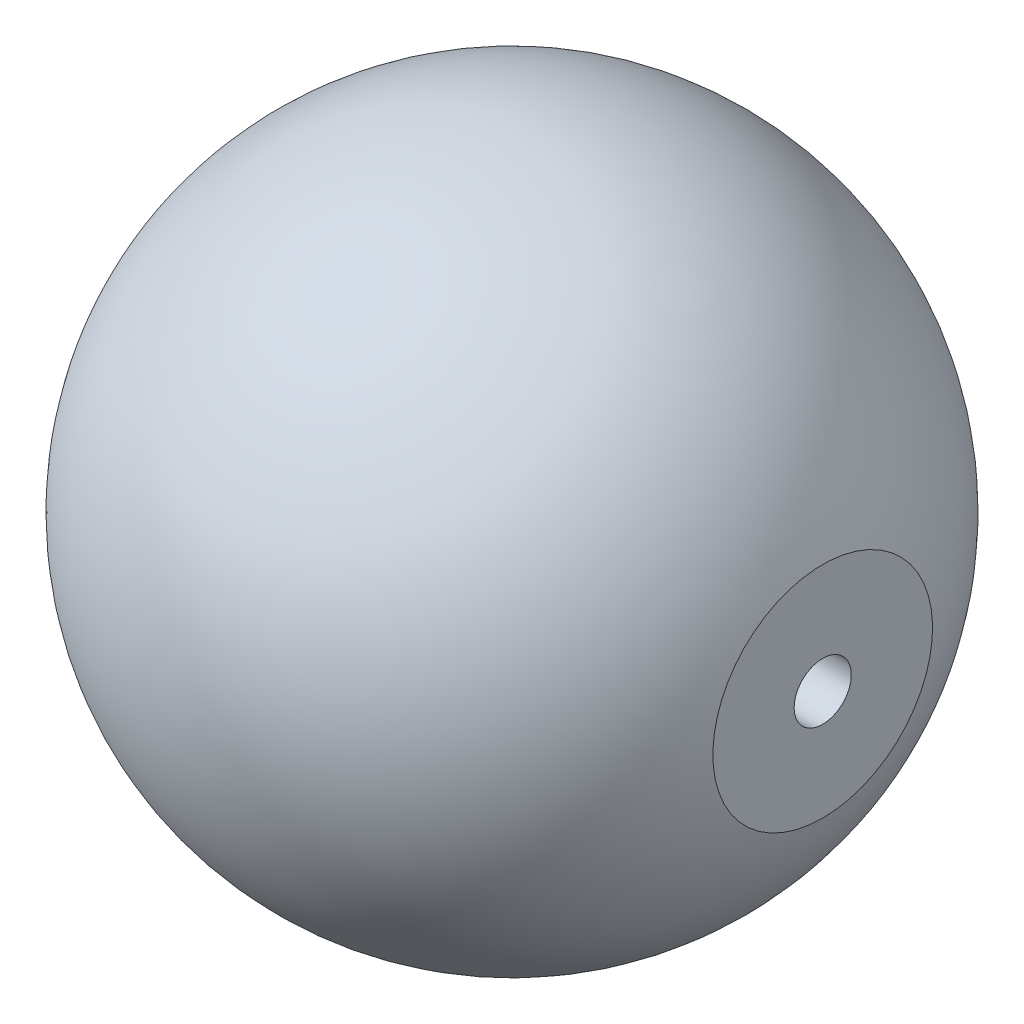
ISO-10303-21;
HEADER;
FILE_DESCRIPTION(('STEP AP214'),'2;1');
FILE_NAME('part.step','',(''),(''),'','','');
FILE_SCHEMA(('AUTOMOTIVE_DESIGN { 1 0 10303 214 1 1 1 1 }'));
ENDSEC;
DATA;
#1=APPLICATION_CONTEXT('core data for automotive mechanical design processes');
#2=APPLICATION_PROTOCOL_DEFINITION('international standard','automotive_design',2000,#1);
#3=PRODUCT_CONTEXT('',#1,'mechanical');
#4=PRODUCT('Part','Part','',(#3));
#5=PRODUCT_RELATED_PRODUCT_CATEGORY('part','',(#4));
#6=PRODUCT_DEFINITION_FORMATION('','',#4);
#7=PRODUCT_DEFINITION_CONTEXT('part definition',#1,'design');
#8=PRODUCT_DEFINITION('design','',#6,#7);
#9=PRODUCT_DEFINITION_SHAPE('','',#8);
#10=(LENGTH_UNIT() NAMED_UNIT(*) SI_UNIT(.MILLI.,.METRE.));
#11=(NAMED_UNIT(*) PLANE_ANGLE_UNIT() SI_UNIT($,.RADIAN.));
#12=(NAMED_UNIT(*) SI_UNIT($,.STERADIAN.) SOLID_ANGLE_UNIT());
#13=UNCERTAINTY_MEASURE_WITH_UNIT(LENGTH_MEASURE(1.E-05),#10,'distance_accuracy_value','');
#14=(GEOMETRIC_REPRESENTATION_CONTEXT(3) GLOBAL_UNCERTAINTY_ASSIGNED_CONTEXT((#13)) GLOBAL_UNIT_ASSIGNED_CONTEXT((#10,
#11,#12)) REPRESENTATION_CONTEXT('',''));
#15=CARTESIAN_POINT('',(0.,0.,0.));
#16=DIRECTION('',(0.,0.,1.));
#17=DIRECTION('',(1.,0.,0.));
#18=AXIS2_PLACEMENT_3D('',#15,#16,#17);
#19=CARTESIAN_POINT('',(-30.,0.,0.));
#20=DIRECTION('',(-1.,0.,0.));
#21=DIRECTION('',(0.,0.,1.));
#22=AXIS2_PLACEMENT_3D('',#19,#20,#21);
#23=CYLINDRICAL_SURFACE('',#22,2.6);
#24=CARTESIAN_POINT('',(-28.2842712474619,0.,0.));
#25=DIRECTION('',(-1.,0.,0.));
#26=DIRECTION('',(0.,0.,1.));
#27=AXIS2_PLACEMENT_3D('',#24,#25,#26);
#28=CIRCLE('',#27,2.6);
#29=CARTESIAN_POINT('',(-28.2842712474619,0.,2.6));
#30=VERTEX_POINT('',#29);
#31=EDGE_CURVE('E10',#30,#30,#28,.T.);
#32=ORIENTED_EDGE('',*,*,#31,.T.);
#33=EDGE_LOOP('',(#32));
#34=FACE_BOUND('',#33,.T.);
#35=CARTESIAN_POINT('',(28.2842712474619,0.,0.));
#36=DIRECTION('',(-1.,0.,0.));
#37=DIRECTION('',(0.,0.,1.));
#38=AXIS2_PLACEMENT_3D('',#35,#36,#37);
#39=CIRCLE('',#38,2.6);
#40=CARTESIAN_POINT('',(28.2842712474619,0.,2.6));
#41=VERTEX_POINT('',#40);
#42=EDGE_CURVE('E51',#41,#41,#39,.T.);
#43=ORIENTED_EDGE('',*,*,#42,.F.);
#44=EDGE_LOOP('',(#43));
#45=FACE_BOUND('',#44,.T.);
#46=ADVANCED_FACE('F40',(#34,#45),#23,.F.);
#47=CARTESIAN_POINT('',(-28.2842712474619,-2.6,0.));
#48=DIRECTION('',(-1.,0.,0.));
#49=DIRECTION('',(0.,0.,1.));
#50=AXIS2_PLACEMENT_3D('',#47,#48,#49);
#51=PLANE('',#50);
#52=CARTESIAN_POINT('',(-28.2842712474619,0.,0.));
#53=DIRECTION('',(-1.,0.,0.));
#54=DIRECTION('',(0.,0.,1.));
#55=AXIS2_PLACEMENT_3D('',#52,#53,#54);
#56=CIRCLE('',#55,10.);
#57=CARTESIAN_POINT('',(-28.2842712474619,-10.,0.));
#58=VERTEX_POINT('',#57);
#59=EDGE_CURVE('E43',#58,#58,#56,.T.);
#60=ORIENTED_EDGE('',*,*,#59,.T.);
#61=EDGE_LOOP('',(#60));
#62=FACE_BOUND('',#61,.T.);
#63=ORIENTED_EDGE('',*,*,#31,.F.);
#64=EDGE_LOOP('',(#63));
#65=FACE_BOUND('',#64,.T.);
#66=ADVANCED_FACE('F62',(#62,#65),#51,.T.);
#67=CARTESIAN_POINT('',(0.,0.,0.));
#68=DIRECTION('',(-1.,0.,0.));
#69=DIRECTION('',(0.,-1.,0.));
#70=AXIS2_PLACEMENT_3D('',#67,#68,#69);
#71=SPHERICAL_SURFACE('',#70,30.);
#72=CARTESIAN_POINT('',(28.2842712474619,0.,0.));
#73=DIRECTION('',(-1.,0.,0.));
#74=DIRECTION('',(0.,0.,1.));
#75=AXIS2_PLACEMENT_3D('',#72,#73,#74);
#76=CIRCLE('',#75,10.);
#77=CARTESIAN_POINT('',(28.2842712474619,-10.,0.));
#78=VERTEX_POINT('',#77);
#79=EDGE_CURVE('E50',#78,#78,#76,.T.);
#80=CARTESIAN_POINT('',(28.2842712474619,-10.,0.));
#81=CARTESIAN_POINT('',(28.1560499634167,-10.3626763441463,0.));
#82=CARTESIAN_POINT('',(28.02084589577,-10.7228836236924,0.));
#83=CARTESIAN_POINT('',(27.7366882806497,-11.4378334803499,0.));
#84=CARTESIAN_POINT('',(27.5877347331762,-11.7925760574612,0.));
#85=CARTESIAN_POINT('',(27.2762942457787,-12.4960699360148,0.));
#86=CARTESIAN_POINT('',(27.1138073058547,-12.8448212374571,0.));
#87=CARTESIAN_POINT('',(26.7755415954182,-13.5358170223894,0.));
#88=CARTESIAN_POINT('',(26.5997628249058,-13.8780615058794,0.));
#89=CARTESIAN_POINT('',(26.2351732206984,-14.5555371593778,0.));
#90=CARTESIAN_POINT('',(26.0463623870035,-14.8907683293863,0.));
#91=CARTESIAN_POINT('',(25.6559880969787,-15.5537213925891,0.));
#92=CARTESIAN_POINT('',(25.4544246406489,-15.8814432857834,0.));
#93=CARTESIAN_POINT('',(25.0388433093674,-16.5288929008077,0.));
#94=CARTESIAN_POINT('',(24.8248254344156,-16.8486206226378,0.));
#95=CARTESIAN_POINT('',(24.3846519251196,-17.4796088394449,0.));
#96=CARTESIAN_POINT('',(24.1584962907753,-17.7908693344219,0.));
#97=CARTESIAN_POINT('',(23.6943818729949,-18.4044625668518,0.));
#98=CARTESIAN_POINT('',(23.4564230895589,-18.7067953043047,0.));
#99=CARTESIAN_POINT('',(22.9690544494358,-19.3020857010117,0.));
#100=CARTESIAN_POINT('',(22.7196445927487,-19.5950433602658,0.));
#101=CARTESIAN_POINT('',(22.2097428240276,-20.1711501507206,0.));
#102=CARTESIAN_POINT('',(21.9492509119935,-20.4542992819213,0.));
#103=CARTESIAN_POINT('',(21.4175704472448,-21.0103700788239,0.));
#104=CARTESIAN_POINT('',(21.1463818945302,-21.2832917445257,0.));
#105=CARTESIAN_POINT('',(20.5937093894201,-21.8185038051668,0.));
#106=CARTESIAN_POINT('',(20.3122254370247,-22.080794200106,0.));
#107=CARTESIAN_POINT('',(19.739378606273,-22.5943556436147,0.));
#108=CARTESIAN_POINT('',(19.4480157279167,-22.8456266921843,0.));
#109=CARTESIAN_POINT('',(18.8558421354703,-23.3367776711817,0.));
#110=CARTESIAN_POINT('',(18.5550314213803,-23.5766576016095,0.));
#111=CARTESIAN_POINT('',(17.9444072263787,-24.0446714264476,0.));
#112=CARTESIAN_POINT('',(17.6345937454672,-24.2728053208579,0.));
#113=CARTESIAN_POINT('',(17.0064224059104,-24.7169895348056,0.));
#114=CARTESIAN_POINT('',(16.6880645472651,-24.9330398543429,0.));
#115=CARTESIAN_POINT('',(16.0432754832885,-25.3527372581198,0.));
#116=CARTESIAN_POINT('',(15.7168442779571,-25.5563843423593,0.));
#117=CARTESIAN_POINT('',(15.0563914966943,-25.9509739665048,0.));
#118=CARTESIAN_POINT('',(14.722369920763,-26.1419165064108,0.));
#119=CARTESIAN_POINT('',(14.0472306048311,-26.5108145300486,0.));
#120=CARTESIAN_POINT('',(13.7061128648305,-26.6887700137805,0.));
#121=CARTESIAN_POINT('',(13.0172859265244,-27.0314306284194,0.));
#122=CARTESIAN_POINT('',(12.6695767282189,-27.1961357593265,0.));
#123=CARTESIAN_POINT('',(11.9680813315563,-27.5120519764192,0.));
#124=CARTESIAN_POINT('',(11.6142951331993,-27.6632630626049,0.));
#125=CARTESIAN_POINT('',(10.9011691860019,-27.9519674636707,0.));
#126=CARTESIAN_POINT('',(10.5418294371615,-28.0894607785507,0.));
#127=CARTESIAN_POINT('',(9.81812805540266,-28.3505262067507,0.));
#128=CARTESIAN_POINT('',(9.45376642248421,-28.4740983200707,0.));
#129=CARTESIAN_POINT('',(8.72056036917696,-28.7071385122147,0.));
#130=CARTESIAN_POINT('',(8.35171594878817,-28.8166065910387,0.));
#131=CARTESIAN_POINT('',(7.61009004972202,-29.0212767490864,0.));
#132=CARTESIAN_POINT('',(7.23730857104466,-29.11647882831,0.));
#133=CARTESIAN_POINT('',(6.48836010971561,-29.2924761295216,0.));
#134=CARTESIAN_POINT('',(6.11219312706391,-29.3732713515096,0.));
#135=CARTESIAN_POINT('',(5.35703022117255,-29.5203353964921,0.));
#136=CARTESIAN_POINT('',(4.97803429793287,-29.5866042194866,0.));
#137=CARTESIAN_POINT('',(4.21777425985254,-29.7045174174715,0.));
#138=CARTESIAN_POINT('',(3.83651014501188,-29.7561617924618,0.));
#139=CARTESIAN_POINT('',(3.07227782865276,-29.8447496832443,0.));
#140=CARTESIAN_POINT('',(2.6893096271343,-29.8816931990365,0.));
#141=CARTESIAN_POINT('',(1.92223576364926,-29.9408247111012,0.));
#142=CARTESIAN_POINT('',(1.53813010168269,-29.9630127073737,0.));
#143=CARTESIAN_POINT('',(0.769349626477406,-29.9926003518231,0.));
#144=CARTESIAN_POINT('',(0.384674813238703,-30.,0.));
#145=CARTESIAN_POINT('',(-0.384674813238703,-30.,0.));
#146=CARTESIAN_POINT('',(-0.769349626477406,-29.9926003518231,0.));
#147=CARTESIAN_POINT('',(-1.53813010168269,-29.9630127073737,0.));
#148=CARTESIAN_POINT('',(-1.92223576364926,-29.9408247111012,0.));
#149=CARTESIAN_POINT('',(-2.6893096271343,-29.8816931990365,0.));
#150=CARTESIAN_POINT('',(-3.07227782865276,-29.8447496832443,0.));
#151=CARTESIAN_POINT('',(-3.83651014501188,-29.7561617924618,0.));
#152=CARTESIAN_POINT('',(-4.21777425985254,-29.7045174174715,0.));
#153=CARTESIAN_POINT('',(-4.97803429793287,-29.5866042194866,0.));
#154=CARTESIAN_POINT('',(-5.35703022117255,-29.5203353964921,0.));
#155=CARTESIAN_POINT('',(-6.11219312706391,-29.3732713515096,0.));
#156=CARTESIAN_POINT('',(-6.48836010971561,-29.2924761295216,0.));
#157=CARTESIAN_POINT('',(-7.23730857104466,-29.11647882831,0.));
#158=CARTESIAN_POINT('',(-7.61009004972202,-29.0212767490864,0.));
#159=CARTESIAN_POINT('',(-8.35171594878817,-28.8166065910387,0.));
#160=CARTESIAN_POINT('',(-8.72056036917696,-28.7071385122147,0.));
#161=CARTESIAN_POINT('',(-9.4537664224842,-28.4740983200707,0.));
#162=CARTESIAN_POINT('',(-9.81812805540266,-28.3505262067507,0.));
#163=CARTESIAN_POINT('',(-10.5418294371615,-28.0894607785507,0.));
#164=CARTESIAN_POINT('',(-10.9011691860019,-27.9519674636707,0.));
#165=CARTESIAN_POINT('',(-11.6142951331993,-27.6632630626049,0.));
#166=CARTESIAN_POINT('',(-11.9680813315563,-27.5120519764192,0.));
#167=CARTESIAN_POINT('',(-12.6695767282189,-27.1961357593265,0.));
#168=CARTESIAN_POINT('',(-13.0172859265244,-27.0314306284194,0.));
#169=CARTESIAN_POINT('',(-13.7061128648305,-26.6887700137805,0.));
#170=CARTESIAN_POINT('',(-14.0472306048311,-26.5108145300486,0.));
#171=CARTESIAN_POINT('',(-14.722369920763,-26.1419165064108,0.));
#172=CARTESIAN_POINT('',(-15.0563914966943,-25.9509739665048,0.));
#173=CARTESIAN_POINT('',(-15.7168442779571,-25.5563843423593,0.));
#174=CARTESIAN_POINT('',(-16.0432754832885,-25.3527372581198,0.));
#175=CARTESIAN_POINT('',(-16.6880645472651,-24.9330398543429,0.));
#176=CARTESIAN_POINT('',(-17.0064224059104,-24.7169895348056,0.));
#177=CARTESIAN_POINT('',(-17.6345937454672,-24.2728053208579,0.));
#178=CARTESIAN_POINT('',(-17.9444072263787,-24.0446714264476,0.));
#179=CARTESIAN_POINT('',(-18.5550314213803,-23.5766576016095,0.));
#180=CARTESIAN_POINT('',(-18.8558421354703,-23.3367776711817,0.));
#181=CARTESIAN_POINT('',(-19.4480157279167,-22.8456266921843,0.));
#182=CARTESIAN_POINT('',(-19.739378606273,-22.5943556436147,0.));
#183=CARTESIAN_POINT('',(-20.3122254370247,-22.080794200106,0.));
#184=CARTESIAN_POINT('',(-20.5937093894201,-21.8185038051668,0.));
#185=CARTESIAN_POINT('',(-21.1463818945302,-21.2832917445257,0.));
#186=CARTESIAN_POINT('',(-21.4175704472448,-21.0103700788239,0.));
#187=CARTESIAN_POINT('',(-21.9492509119935,-20.4542992819213,0.));
#188=CARTESIAN_POINT('',(-22.2097428240276,-20.1711501507206,0.));
#189=CARTESIAN_POINT('',(-22.7196445927487,-19.5950433602658,0.));
#190=CARTESIAN_POINT('',(-22.9690544494358,-19.3020857010117,0.));
#191=CARTESIAN_POINT('',(-23.4564230895589,-18.7067953043047,0.));
#192=CARTESIAN_POINT('',(-23.6943818729949,-18.4044625668518,0.));
#193=CARTESIAN_POINT('',(-24.1584962907753,-17.7908693344219,0.));
#194=CARTESIAN_POINT('',(-24.3846519251196,-17.4796088394449,0.));
#195=CARTESIAN_POINT('',(-24.8248254344156,-16.8486206226378,0.));
#196=CARTESIAN_POINT('',(-25.0388433093674,-16.5288929008077,0.));
#197=CARTESIAN_POINT('',(-25.4544246406489,-15.8814432857834,0.));
#198=CARTESIAN_POINT('',(-25.6559880969788,-15.5537213925891,0.));
#199=CARTESIAN_POINT('',(-26.0463623870035,-14.8907683293863,0.));
#200=CARTESIAN_POINT('',(-26.2351732206984,-14.5555371593778,0.));
#201=CARTESIAN_POINT('',(-26.5997628249058,-13.8780615058794,0.));
#202=CARTESIAN_POINT('',(-26.7755415954182,-13.5358170223894,0.));
#203=CARTESIAN_POINT('',(-27.1138073058547,-12.8448212374571,0.));
#204=CARTESIAN_POINT('',(-27.2762942457787,-12.4960699360149,0.));
#205=CARTESIAN_POINT('',(-27.5877347331762,-11.7925760574612,0.));
#206=CARTESIAN_POINT('',(-27.7366882806497,-11.4378334803499,0.));
#207=CARTESIAN_POINT('',(-28.02084589577,-10.7228836236924,0.));
#208=CARTESIAN_POINT('',(-28.1560499634167,-10.3626763441463,0.));
#209=CARTESIAN_POINT('',(-28.2842712474619,-10.,0.));
#210=B_SPLINE_CURVE_WITH_KNOTS('',3,(#80,#81,#82,#83,#84,#85,#86,#87,#88,#89,#90,#91,#92,#93,
#94,#95,#96,#97,#98,#99,#100,#101,#102,#103,#104,#105,#106,#107,#108,#109,#110,#111,#112,#113,
#114,#115,#116,#117,#118,#119,#120,#121,#122,#123,#124,#125,#126,#127,#128,#129,#130,#131,#132,
#133,#134,#135,#136,#137,#138,#139,#140,#141,#142,#143,#144,#145,#146,#147,#148,#149,#150,#151,
#152,#153,#154,#155,#156,#157,#158,#159,#160,#161,#162,#163,#164,#165,#166,#167,#168,#169,#170,
#171,#172,#173,#174,#175,#176,#177,#178,#179,#180,#181,#182,#183,#184,#185,#186,#187,#188,#189,
#190,#191,#192,#193,#194,#195,#196,#197,#198,#199,#200,#201,#202,#203,#204,#205,#206,#207,#208,
#209),.UNSPECIFIED.,.F.,.F.,(4,2,2,2,2,2,2,2,2,2,2,2,2,2,2,2,2,2,2,2,2,2,2,2,2,2,2,2,2,2,2,2,2,
2,2,2,2,2,2,2,2,2,2,2,2,2,2,2,2,2,2,2,2,2,2,2,2,2,2,2,2,2,2,2,4),(0.,1.15395330238962,
2.30790660477923,3.46185990716885,4.61581320955847,5.76976651194809,6.9237198143377,
8.07767311672732,9.23162641911694,10.3855797215066,11.5395330238962,12.6934863262858,
13.8474396286754,15.001392931065,16.1553462334546,17.3092995358443,18.4632528382339,
19.6172061406235,20.7711594430131,21.9251127454027,23.0790660477923,24.233019350182,
25.3869726525716,26.5409259549612,27.6948792573508,28.8488325597404,30.0027858621301,
31.1567391645197,32.3106924669093,33.4646457692989,34.6185990716885,35.7725523740781,
36.9265056764677,38.0804589788574,39.234412281247,40.3883655836366,41.5423188860262,
42.6962721884158,43.8502254908054,45.0041787931951,46.1581320955847,47.3120853979743,
48.4660387003639,49.6199920027535,50.7739453051432,51.9278986075328,53.0818519099224,
54.235805212312,55.3897585147016,56.5437118170912,57.6976651194808,58.8516184218705,
60.0055717242601,61.1595250266497,62.3134783290393,63.4674316314289,64.6213849338186,
65.7753382362082,66.9292915385978,68.0832448409874,69.237198143377,70.3911514457666,
71.5451047481562,72.6990580505459,73.8530113529355),.UNSPECIFIED.);
#211=EDGE_CURVE('BSEAM63',#78,#58,#210,.T.);
#212=ORIENTED_EDGE('',*,*,#79,.T.);
#213=ORIENTED_EDGE('',*,*,#59,.F.);
#214=ORIENTED_EDGE('',*,*,#211,.T.);
#215=ORIENTED_EDGE('',*,*,#211,.F.);
#216=EDGE_LOOP('',(#212,#214,#213,#215));
#217=FACE_BOUND('',#216,.T.);
#218=ADVANCED_FACE('F63',(#217),#71,.T.);
#219=CARTESIAN_POINT('',(28.2842712474619,-2.6,0.));
#220=DIRECTION('',(1.,0.,0.));
#221=DIRECTION('',(0.,0.,-1.));
#222=AXIS2_PLACEMENT_3D('',#219,#220,#221);
#223=PLANE('',#222);
#224=ORIENTED_EDGE('',*,*,#42,.T.);
#225=EDGE_LOOP('',(#224));
#226=FACE_BOUND('',#225,.T.);
#227=ORIENTED_EDGE('',*,*,#79,.F.);
#228=EDGE_LOOP('',(#227));
#229=FACE_BOUND('',#228,.T.);
#230=ADVANCED_FACE('F60',(#226,#229),#223,.T.);
#231=CLOSED_SHELL('',(#46,#66,#218,#230));
#232=MANIFOLD_SOLID_BREP('B2',#231);
#233=ADVANCED_BREP_SHAPE_REPRESENTATION('',(#18,#232),#14);
#234=SHAPE_DEFINITION_REPRESENTATION(#9,#233);
ENDSEC;
END-ISO-10303-21;
